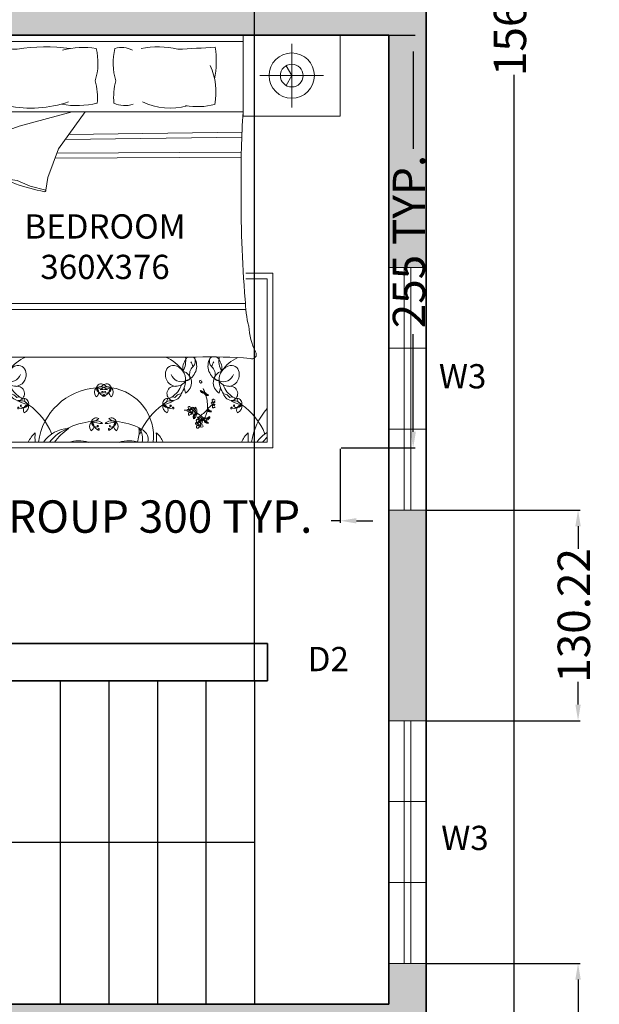
# Model space of a CAD drawing. Units: centimetres. Extents: x 2137 to 3697, y 183 to 2094.
# Tile 6 of 8: x 3339 to 3697, y 600 to 1208. Entities that reach past the tile are written whole.
import ezdxf

# ---------------------------------------------------------------- set-up
doc = ezdxf.new("R2010")
doc.units = ezdxf.units.CM
for name, color, linetype, lineweight in [('A-ANNO-DIMS', 2, 'Continuous', 18), ('A-ANNO-TEXT', 7, 'Continuous', 18), ('A-AREA-IDEN', 7, 'Continuous', 25), ('A-FLOR-STRS', 7, 'Continuous', 25), ('A-FURN', 8, 'Continuous', 18), ('A-GLAZ', 4, 'Continuous', 18), ('A-WALL', 7, 'Continuous', 35), ('A-WALL-PATT', 52, 'Continuous', 13)]:
    doc.layers.add(name, color=color, linetype=linetype, lineweight=lineweight)
doc.styles.get("Standard").update_dxf_attribs({"font": 'arial.ttf'})
doc.dimstyles.new('ISO-25', dxfattribs={"dimtxt": 20, "dimasz": 10, "dimexe": 1.25, "dimexo": 0.625, "dimtad": 0, "dimtxsty": 'Standard', "dimcen": 2.5, "dimadec": 0, "dimazin": 0, "dimtfac": 1, "dimtmove": 0, "dimatfit": 3, "dimfxl": 1, "dimarcsym": 0})

# ---------------------------------------------------------------- blocks, each defined once
blk = doc.blocks.new('*D3')
at = {"layer": 'A-ANNO-DIMS', "color": 0, "lineweight": -2, "transparency": 16777216}
for p, q in [((3590.65, 1986.58), (3645.66, 1986.58)), ((3644.41, 1976.58), (3644.41, 1233.12)), ((3644.41, 430.58), (3644.41, 1174.04)), ((3590.65, 420.58), (3645.66, 420.58))]:
    blk.add_line(p, q, dxfattribs=at)
at = {"layer": 'A-ANNO-DIMS', "color": 0, "transparency": 16777216}
for points in [[(3642.74, 1976.58), (3646.07, 1976.58), (3644.41, 1986.58)], [(3642.74, 430.58), (3646.07, 430.58), (3644.41, 420.58)]]:
    blk.add_solid(points, dxfattribs=at)
at = {"layer": 'Defpoints', "color": 0, "transparency": 16777216}
for p in [(3590.02, 1986.58), (3644.41, 1986.58), (3590.02, 420.58)]:
    blk.add_point(p, dxfattribs=at)
at = {"layer": 'A-ANNO-DIMS', "color": 0, "transparency": 16777216, "insert": (3644.41, 1203.58), "char_height": 20, "attachment_point": 5, "rotation": 90}
blk.add_mtext('1566', dxfattribs=at)
blk = doc.blocks.new('BED')
for p, q in [((2442.52, 2474.71), (2742.52, 2474.71)), ((2502.52, 2474.71), (2502.52, 2392.37)), ((2682.52, 2470.86), (2502.52, 2470.86)), ((2472.52, 2430.11), (2472.52, 2469.31)), ((2712.52, 2430.11), (2712.52, 2469.31)), ((2492.12, 2449.71), (2452.92, 2449.71)), ((2692.92, 2449.71), (2732.12, 2449.71)), ((2502.52, 2427.3), (2682.52, 2427.3)), ((2544.19, 2418.38), (2576.9, 2427.3)), ((2584.93, 2427.3), (2568.49, 2404.42)), ((2522.31, 2410.49), (2544.19, 2418.38)), ((2510.77, 2401.99), (2522.31, 2410.49)), ((2681.6, 2411.76), (2572.66, 2410.22)), ((2681.71, 2414.84), (2574.9, 2413.34)), ((2568.49, 2404.42), (2561.81, 2386.81)), ((2499.83, 2389.24), (2510.77, 2401.99)), ((2681.46, 2399.23), (2566.35, 2398.76)), ((2681.44, 2402.31), (2567.52, 2401.86)), ((2502.26, 2386.81), (2499.83, 2389.24)), ((2514.41, 2388.02), (2502.26, 2386.81)), ((2529.61, 2386.81), (2514.41, 2388.02)), ((2542.97, 2384.99), (2529.61, 2386.81)), ((2561.81, 2386.81), (2560.59, 2378.91)), ((2550.87, 2381.34), (2542.97, 2384.99)), ((2560.59, 2378.91), (2550.87, 2381.34)), ((2482.11, 2327.65), (2499.08, 2327.65)), ((2482.11, 2219.58), (2482.11, 2327.65)), ((2684.19, 2327.65), (2700.83, 2327.65)), ((2700.83, 2327.65), (2700.83, 2219.58)), ((2499.08, 2324.17), (2485.59, 2324.17)), ((2485.59, 2324.17), (2485.59, 2223.06)), ((2697.35, 2324.17), (2684.13, 2324.17)), ((2697.35, 2223.06), (2697.35, 2324.17)), ((2683.88, 2308.94), (2499.06, 2308.94)), ((2684.17, 2305.2), (2499.06, 2305.2)), ((2653.42, 2275.73), (2531.62, 2275.73)), ((2515.15, 2253.47), (2514.49, 2256.86)), ((2536.12, 2253.47), (2536.78, 2256.86)), ((2646.82, 2253.47), (2646.16, 2256.86)), ((2667.79, 2253.47), (2668.45, 2256.86)), ((2485.59, 2223.06), (2697.35, 2223.06)), ((2700.83, 2219.58), (2482.11, 2219.58))]:
    blk.add_line(p, q)
for points in [[(2502.52, 2424.71), (2442.52, 2424.71), (2442.52, 2474.71)], [(2682.52, 2474.71), (2682.52, 2424.71), (2742.52, 2424.71), (2742.52, 2474.71)], [(2472.52, 2449.71), (2476.02, 2455.77)], [(2712.52, 2449.71), (2709.02, 2455.77)], [(2472.52, 2449.71), (2476.02, 2443.65)], [(2712.52, 2449.71), (2709.02, 2443.65)]]:
    blk.add_lwpolyline(points)
for points in [[(2519.75, 2467.23, 0.074897), (2520.11, 2447.64, -0.472817)], [(2591.11, 2446.54, 0.14099), (2591.71, 2466.53, 0.235245)], [(2603.92, 2446.54, -0.14099), (2603.32, 2466.53, -0.235245)], [(2665.29, 2467.23, -0.074897), (2664.92, 2447.64, 0.472817)], [(2499.2, 2361.77, 0.001242), (2499.06, 2304.85, -0.127202), (2493.05, 2276.48)], [(2683.8, 2311.3, 0.056112), (2685.97, 2294.79, 0.095341), (2690.19, 2278.9)]]:
    blk.add_lwpolyline(points, format="xyb")
for centre, radius in [((2472.52, 2449.71), 14), ((2712.52, 2449.71), 14), ((2472.52, 2449.71), 7), ((2712.52, 2449.71), 7), ((2532.49, 2242.6), 0.764), ((2650.46, 2242.6), 0.764), ((2527.49, 2234.55), 0.764), ((2655.45, 2234.55), 0.764)]:
    blk.add_circle(centre, radius)
for centre, radius, start, end in [((2685.11, 5322.24), 2859.79, 266.68521, 267.14978), ((2560.85, 2358.67), 108.8, 82.21958, 99.49698), ((2583.83, 2413.66), 53.46, 81.52493, 103.95996), ((2607.44, 2452.27), 14.84, 63.34374, 106.10256), ((2629.68, 2414.74), 52.74, 76.34271, 101.1841), ((2499.93, 5322.24), 2859.79, 272.85022, 273.31479), ((2557.97, 2439.77), 38.67, 155.1316, 191.75834), ((2627.07, 2439.77), 38.67, 348.24166, 24.8684), ((2555.75, 2436.51), 36.76, 354.01289, 15.82928), ((2639.29, 2436.51), 36.76, 164.17072, 185.98711), ((2530.45, 2470.74), 40.2, 255.10393, 281.03689), ((2551.61, 2499.32), 69.73, 258.03974, 289.26152), ((2579.84, 2484.1), 52.9, 259.86169, 283.62376), ((2609.45, 2447.1), 15.9, 245.01826, 288.54073), ((2637.23, 2467.78), 38.19, 243.87611, 286.17464), ((2654.58, 2470.74), 40.2, 258.96311, 284.89607), ((3220.32, 2390.64), 539.05, 176.09997, 180.92818), ((2224.76, 2381.78), 275.17, 355.82941, 1.55305), ((2504.97, 2495.47), 113.22, 267.45188, 281.3392), ((2532.03, 2360.52), 24.42, 66.26158, 101.3392), ((2581.42, 2492.28), 116.34, 250.11942, 259.33829), ((3384.42, 2371.04), 703.17, 179.11454, 184.87351), ((2559.91, 2378.67), 0.724, 268.86235, 19.75363), ((2495.81, 2276.67), 2.77, 183.97998, 297.34124), ((2687.92, 2277.37), 2.73, 246.52186, 33.82642), ((2528.04, 1963.45), 312.3, 89.34325, 95.68869), ((2507.86, 2265.5), 5.07, 84.48557, 181.05378), ((2494.64, 2254.6), 22.71, 33.66712, 63.29966), ((2506.31, 2261.76), 9.02, 355.29334, 76.921), ((2525.07, 2268.11), 11.57, 145.78505, 184.73037), ((2502.97, 2273.51), 12.43, 328.82178, 9.15542), ((2518.36, 2272.41), 3.61, 120.0293, 142.32497), ((2512.59, 2270.28), 9.56, 289.28218, 29.1751), ((2511.15, 2268.55), 8.62, 7.43599, 29.91487), ((2516.83, 2273.13), 4.49, 311.56531, 23.83541), ((2518.36, 2272.41), 3.61, 44.45169, 63.55801), ((2538.68, 2270.28), 9.56, 150.8249, 250.71782), ((2534.44, 2273.13), 4.49, 156.16459, 228.43469), ((2532.91, 2272.41), 3.61, 113.22901, 135.54831), ((2540.13, 2268.55), 8.62, 150.08513, 172.56401), ((2532.91, 2272.41), 3.61, 37.67503, 66.71436), ((2526.21, 2268.11), 11.57, 355.26963, 34.21495), ((2548.31, 2273.51), 12.43, 169.71335, 211.17822), ((2544.97, 2261.76), 9.02, 103.079, 184.70666), ((2556.64, 2254.6), 22.71, 111.49413, 146.33288), ((2543.41, 2265.5), 5.07, 358.94622, 95.51443), ((2639.53, 2265.5), 5.07, 84.48557, 181.05378), ((2626.3, 2254.6), 22.71, 33.66712, 68.50587), ((2637.98, 2261.76), 9.02, 355.29334, 76.921), ((2656.73, 2268.11), 11.57, 145.78505, 184.73037), ((2634.63, 2273.51), 12.43, 328.82178, 10.28665), ((2650.03, 2272.41), 3.61, 113.28564, 142.32497), ((2644.26, 2270.28), 9.56, 289.28218, 29.1751), ((2642.81, 2268.55), 8.62, 7.43599, 29.91487), ((2650.03, 2272.41), 3.61, 44.45169, 66.71436), ((2648.5, 2273.13), 4.49, 311.56531, 23.83541), ((2662.61, 1983.95), 291.92, 85.24024, 91.80351), ((2670.35, 2270.28), 9.56, 150.8249, 250.71782), ((2666.11, 2273.13), 4.49, 156.16459, 228.43469), ((2664.58, 2272.41), 3.61, 106.63434, 135.54831), ((2671.79, 2268.55), 8.62, 150.08513, 172.56401), ((2664.58, 2272.41), 3.61, 37.67503, 72.58143), ((2657.87, 2268.11), 11.57, 355.26963, 34.21495), ((2679.98, 2273.51), 12.43, 169.24899, 211.17822), ((2676.63, 2261.76), 9.02, 103.079, 184.70666), ((2688.3, 2254.6), 22.71, 113.64533, 146.33288), ((2675.08, 2265.5), 5.07, 358.94622, 95.51443), ((2509.94, 2264.78), 7.17, 174.94485, 262.88575), ((2512.76, 2267.5), 6.96, 201.58187, 291.42215), ((2511.44, 2259.94), 7.46, 299.90854, 73.1337), ((2523.89, 2265.16), 6.15, 131.56531, 195.14713), ((2527.38, 2265.16), 6.15, 344.85287, 48.43469), ((2539.84, 2259.94), 7.46, 106.8663, 240.09146), ((2538.52, 2267.5), 6.96, 248.57785, 338.41813), ((2541.33, 2264.78), 7.17, 277.11425, 5.05515), ((2641.61, 2264.78), 7.17, 174.94485, 262.88575), ((2644.43, 2267.5), 6.96, 201.58187, 291.42215), ((2643.1, 2259.94), 7.46, 299.90854, 73.1337), ((2655.56, 2265.16), 6.15, 131.56531, 195.14713), ((2659.05, 2265.16), 6.15, 344.85287, 48.43469), ((2671.51, 2259.94), 7.46, 106.8663, 240.09146), ((2670.18, 2267.5), 6.96, 248.57785, 338.41813), ((2673, 2264.78), 7.17, 277.11425, 5.05515), ((2499.37, 2263.14), 14.16, 301.26137, 341.7045), ((2508.7, 2266.37), 8.71, 272.3591, 324.04014), ((2499.23, 2262), 16.1, 326.28828, 356.5076), ((2525.07, 2268.11), 11.57, 212.70113, 216.34448), ((2516.16, 2263.07), 1.86, 257.30406, 15.14713), ((2526.5, 2260.25), 0.578, 102.70507, 280.43845), ((2526.43, 2260.6), 0.94, 280.43845, 100.41356), ((2535.12, 2263.07), 1.86, 164.85287, 282.69594), ((2526.21, 2268.11), 11.57, 323.65552, 327.29887), ((2542.58, 2266.37), 8.71, 215.95986, 267.6409), ((2552.04, 2262), 16.1, 183.4924, 213.71172), ((2551.91, 2263.14), 14.16, 198.2955, 238.73863), ((2594.92, 2255.93), 3.25, 63.02737, 163.80375), ((2591.63, 2263.52), 6.69, 271.45846, 315.37266), ((2598.02, 2255.93), 3.25, 16.19625, 116.97263), ((2601.31, 2263.52), 6.69, 224.62734, 268.54154), ((2631.03, 2263.14), 14.16, 301.26137, 341.7045), ((2640.36, 2266.37), 8.71, 272.3591, 324.04014), ((2630.9, 2262), 16.1, 326.28828, 356.5076), ((2656.73, 2268.11), 11.57, 212.70113, 216.34448), ((2647.82, 2263.07), 1.86, 257.30406, 15.14713), ((2656.51, 2260.6), 0.94, 79.58644, 259.56155), ((2656.44, 2260.25), 0.578, 259.56155, 77.29493), ((2666.78, 2263.07), 1.86, 164.85287, 282.69594), ((2657.87, 2268.11), 11.57, 323.65552, 327.29887), ((2674.25, 2266.37), 8.71, 215.95986, 267.6409), ((2683.71, 2262), 16.1, 183.4924, 213.71172), ((2683.58, 2263.14), 14.16, 198.2955, 238.73863), ((2508.29, 2253.23), 4.5, 80.26398, 250.86884), ((2507.21, 2254.58), 5.62, 265.96902, 344.3045), ((2513.27, 2247.11), 5.99, 96.1662, 141.58255), ((2523.19, 2251.31), 1.58, 101.32561, 154.46214), ((2520.92, 2256.65), 4.74, 280.25878, 300.65599), ((2522.01, 2260.45), 8.46, 268.32639, 277.13024), ((2547.29, 2245.15), 24.85, 163.58418, 183.82768), ((2519.89, 2256.64), 4.82, 308.21012, 316.30712), ((2522.85, 2253.47), 1.44, 278.34322, 4.28685), ((2522.06, 2254.74), 2.51, 300.65599, 332.63414), ((2523.94, 2253.08), 0.611, 55.76575, 157.44165), ((2547.29, 2245.15), 24.85, 153.0032, 159.89408), ((2524.9, 2253.65), 0.611, 84.37838, 186.05427), ((2524.32, 2256.1), 2.51, 269.18588, 301.16403), ((2525.06, 2254.8), 1.44, 237.53317, 323.47681), ((2523.67, 2258.9), 4.82, 285.51291, 293.60991), ((2526.81, 2253.48), 1.58, 87.35788, 140.49441), ((2523.17, 2258), 4.74, 301.16403, 321.56124), ((2519.31, 2258.83), 8.46, 324.68979, 333.49364), ((2538.01, 2247.11), 5.99, 38.41745, 83.8338), ((2544.06, 2254.58), 5.62, 195.6955, 274.03098), ((2542.98, 2253.23), 4.5, 289.13116, 99.73602), ((2594.85, 2217.78), 39.18, 94.46233, 172.25504), ((2595.02, 2253.92), 4.34, 137.78732, 219.11446), ((2590.09, 2254.05), 3.27, 298.5391, 58.36268), ((2594.35, 2251.19), 6.19, 45.54113, 114.31008), ((2600, 2282.98), 27.41, 252.59304, 267.25817), ((2595, 2256.71), 3.2, 177.75849, 283.85198), ((2601.17, 2260.05), 9.91, 198.91595, 238.01098), ((2598.59, 2251.19), 6.19, 65.68992, 134.45887), ((2592.94, 2282.98), 27.41, 272.74183, 287.40696), ((2595.67, 2254.01), 0.424, 283.85198, 219.92454), ((2596.18, 2252.06), 0.487, 238.01098, 71.55918), ((2596.26, 2252.29), 0.236, 71.55918, 188.01668), ((2596.76, 2252.06), 0.487, 108.44082, 301.98902), ((2596.68, 2252.29), 0.236, 351.98332, 108.44082), ((2597.23, 2254.17), 0.255, 320.19092, 256.02088), ((2591.77, 2260.05), 9.91, 301.98902, 341.08405), ((2597.94, 2256.71), 3.2, 256.14802, 2.24151), ((2602.86, 2254.05), 3.27, 121.63732, 241.4609), ((2597.92, 2253.92), 4.34, 320.88554, 42.21268), ((2596.83, 2226.82), 30.32, 352.86355, 81.81966), ((2639.96, 2253.23), 4.5, 80.26398, 250.86884), ((2638.88, 2254.58), 5.62, 265.96902, 344.3045), ((2644.93, 2247.11), 5.99, 96.1662, 141.58255), ((2656.13, 2253.48), 1.58, 39.50559, 92.64212), ((2659.77, 2258), 4.74, 218.43876, 238.83597), ((2663.63, 2258.83), 8.46, 206.50636, 215.31021), ((2657.88, 2254.8), 1.44, 216.52319, 302.46683), ((2658.62, 2256.1), 2.51, 238.83597, 270.81412), ((2659.27, 2258.9), 4.82, 246.39009, 254.48709), ((2635.65, 2245.15), 24.85, 20.10592, 26.9968), ((2658.05, 2253.65), 0.611, 353.94573, 95.62162), ((2659, 2253.08), 0.611, 22.55835, 124.23425), ((2660.09, 2253.47), 1.44, 175.71315, 261.65678), ((2660.89, 2254.74), 2.51, 207.36586, 239.34401), ((2635.65, 2245.15), 24.85, 356.17232, 16.41582), ((2663.05, 2256.64), 4.82, 223.69288, 231.78988), ((2662.02, 2256.65), 4.74, 239.34401, 259.74122), ((2660.93, 2260.45), 8.46, 262.86976, 271.67361), ((2659.76, 2251.31), 1.58, 25.53786, 78.67439), ((2675.73, 2254.58), 5.62, 195.6955, 274.03098), ((2669.67, 2247.11), 5.99, 38.41745, 83.8338), ((2674.65, 2253.23), 4.5, 289.13116, 99.73602), ((2523.45, 2213.9), 39.18, 124.38655, 158.59079), ((2505.57, 2245.31), 4.34, 167.71153, 249.03868), ((2504.48, 2247), 3.25, 92.95159, 193.72796), ((2497.84, 2251.95), 6.69, 301.38267, 345.29688), ((2506.35, 2242.61), 6.19, 75.46535, 144.23429), ((2495.38, 2272.99), 27.41, 282.51726, 297.18239), ((2501.23, 2242.96), 3.27, 328.46331, 88.28689), ((2507.84, 2253.69), 9.91, 228.84017, 267.9352), ((2504.16, 2247.72), 3.2, 207.6827, 313.77619), ((2507.37, 2248.35), 2.76, 63.97555, 143.26805), ((2506.09, 2245.71), 0.424, 313.77619, 249.71835), ((2518.73, 2248.32), 1.27, 101.56373, 142.6358), ((2517.68, 2247.14), 0.764, 273.27684, 86.72316), ((2518.57, 2247.86), 0.73, 91.10805, 181.86747), ((2520.08, 2247.41), 2.32, 203.42757, 227.61037), ((2519.34, 2246.4), 1.58, 80.3487, 133.65382), ((2519.06, 2247.7), 1.25, 229.78892, 317.67915), ((2517.71, 2249.32), 1.84, 288.72627, 352.50315), ((2517.65, 2245.06), 1.78, 355.05304, 68.36176), ((2519.04, 2244.75), 2.5, 83.08516, 105.71709), ((2518.96, 2249.23), 0.59, 345.23556, 144.9248), ((2501.72, 2224.01), 28.48, 43.15413, 52.0459), ((2519.5, 2247.3), 0.658, 317.67915, 80.3487), ((2543.91, 2248.35), 2.76, 36.73195, 116.02445), ((2544.93, 2242.61), 6.19, 35.76571, 104.53465), ((2555.89, 2272.99), 27.41, 242.81761, 257.48274), ((2543.43, 2253.69), 9.91, 272.0648, 311.15983), ((2547.11, 2247.72), 3.2, 226.22381, 332.3173), ((2545.24, 2245.88), 0.255, 290.26671, 226.22708), ((2550.05, 2242.96), 3.27, 91.71311, 211.53669), ((2546.8, 2247), 3.25, 346.27204, 87.04841), ((2553.44, 2251.95), 6.69, 194.70312, 238.61733), ((2545.71, 2245.31), 4.34, 290.96132, 12.28847), ((2527.83, 2213.9), 39.18, 21.40921, 55.61345), ((2655.12, 2213.9), 39.18, 124.38655, 158.59079), ((2637.23, 2245.31), 4.34, 167.71153, 249.03868), ((2636.14, 2247), 3.25, 92.95159, 193.72796), ((2629.51, 2251.95), 6.69, 301.38267, 345.29688), ((2638.02, 2242.61), 6.19, 75.46535, 144.23429), ((2627.05, 2272.99), 27.41, 282.51726, 297.18239), ((2635.83, 2247.72), 3.2, 207.6827, 313.77619), ((2639.51, 2253.69), 9.91, 228.84017, 267.9352), ((2632.89, 2242.96), 3.27, 328.46331, 88.28689), ((2639.03, 2248.35), 2.76, 63.97555, 143.26805), ((2637.75, 2245.71), 0.424, 313.77619, 249.71835), ((2681.22, 2224.01), 28.48, 127.9541, 136.84587), ((2663.45, 2247.3), 0.658, 99.6513, 222.32085), ((2663.88, 2247.7), 1.25, 222.32085, 310.21108), ((2663.6, 2246.4), 1.58, 46.34618, 99.6513), ((2663.98, 2249.23), 0.59, 35.0752, 194.76444), ((2665.23, 2249.32), 1.84, 187.49685, 251.27373), ((2665.29, 2245.06), 1.78, 111.63824, 184.94696), ((2663.9, 2244.75), 2.5, 74.28291, 96.91484), ((2664.38, 2247.86), 0.73, 358.13253, 88.89195), ((2662.86, 2247.41), 2.32, 312.38963, 336.57243), ((2664.21, 2248.32), 1.27, 37.3642, 78.43627), ((2665.27, 2247.14), 0.764, 93.27684, 266.72316), ((2675.58, 2248.35), 2.76, 36.73195, 116.02445), ((2676.59, 2242.61), 6.19, 35.76571, 104.53465), ((2687.56, 2272.99), 27.41, 242.81761, 257.48274), ((2675.1, 2253.69), 9.91, 272.0648, 311.15983), ((2678.78, 2247.72), 3.2, 226.22381, 332.3173), ((2676.9, 2245.88), 0.255, 290.26671, 226.22708), ((2681.72, 2242.96), 3.27, 91.71311, 211.53669), ((2685.1, 2251.95), 6.69, 194.70312, 238.61733), ((2678.46, 2247), 3.25, 346.27204, 87.04841), ((2677.37, 2245.31), 4.34, 290.96132, 12.28847), ((2659.49, 2213.9), 39.18, 21.40921, 55.61345), ((2456.43, 2217.78), 39.18, 7.74496, 41.8856), ((2507.46, 2244.52), 0.236, 101.4834, 217.94089), ((2507.5, 2244.28), 0.487, 267.9352, 101.4834), ((2518.72, 2245.73), 1.26, 217.76209, 259.04026), ((2518.83, 2244.95), 0.586, 232.47371, 355.05304), ((2521.4, 2241.21), 1.58, 101.32561, 154.46214), ((2519.13, 2246.56), 4.74, 280.25878, 300.65599), ((2520.22, 2250.35), 8.46, 268.32639, 277.13024), ((2518.11, 2246.55), 4.82, 308.21012, 316.30712), ((2521.07, 2243.38), 1.44, 278.34322, 4.28685), ((2520.27, 2244.64), 2.51, 300.65599, 332.63414), ((2522.16, 2242.98), 0.611, 55.76575, 157.44165), ((2534.91, 2244.52), 12.46, 184.75602, 209.20408), ((2552.85, 2271.04), 40.99, 222.24124, 232.17444), ((2536.2, 2227.98), 14.94, 120.54402, 139.81798), ((2528.5, 2242.96), 2.12, 272.84988, 356.12261), ((2526.64, 2243.74), 3.48, 304.53686, 16.36991), ((2527, 2242.14), 2.05, 321.76073, 7.92519), ((2527.43, 2239.19), 2.05, 8.72271, 54.88717), ((2527.54, 2237.55), 3.48, 0.278, 72.11105), ((2531.47, 2242.76), 2.46, 127.31045, 187.92519), ((2529.1, 2238.83), 2.12, 20.5253, 88.5375), ((2528.09, 2243.04), 2.53, 355.01064, 41.65801), ((2530.88, 2241.17), 0.757, 148.0499, 225.62681), ((2536.2, 2227.98), 14.94, 113.05007, 113.84774), ((2532.28, 2240.29), 2.41, 104.75581, 148.0499), ((2530.93, 2242.02), 1.51, 247.40857, 351.43859), ((2531.64, 2243.66), 1.04, 126.10456, 271.42811), ((2528.73, 2238.64), 2.53, 334.9899, 21.63727), ((2531.53, 2243.95), 0.749, 353.75256, 131.70535), ((2531.35, 2241.96), 0.506, 262.90601, 7.13198), ((2530.82, 2243.06), 1.05, 0.06451, 61.15075), ((2531.07, 2243.95), 1.2, 311.84125, 355.78771), ((2533.54, 2243.78), 1.27, 101.56373, 176.36503), ((2533.53, 2241.19), 1.26, 151.21959, 259.04026), ((2533.38, 2243.32), 0.73, 91.10805, 181.86747), ((2534.89, 2242.87), 2.32, 203.42757, 227.61037), ((2534.15, 2241.86), 1.58, 80.3487, 133.65382), ((2533.87, 2243.16), 1.25, 229.78892, 317.67915), ((2532.52, 2244.78), 1.84, 288.72627, 352.50315), ((2532.46, 2240.51), 1.78, 355.05304, 68.36176), ((2533.85, 2240.21), 2.5, 83.08516, 105.71709), ((2533.77, 2244.69), 0.59, 345.23556, 144.9248), ((2533.64, 2240.41), 0.586, 232.47371, 355.05304), ((2534.31, 2242.76), 0.658, 317.67915, 80.3487), ((2536.2, 2227.98), 14.94, 87.10709, 94.75853), ((2543.77, 2244.28), 0.487, 78.5166, 272.0648), ((2543.82, 2244.52), 0.236, 322.05911, 78.5166), ((2639.12, 2244.52), 0.236, 101.4834, 217.94089), ((2639.17, 2244.28), 0.487, 267.9352, 101.4834), ((2646.75, 2227.98), 14.94, 85.24147, 92.89291), ((2648.64, 2242.76), 0.658, 99.6513, 222.32085), ((2649.07, 2243.16), 1.25, 222.32085, 310.21108), ((2648.79, 2241.86), 1.58, 46.34618, 99.6513), ((2649.17, 2244.69), 0.59, 35.0752, 194.76444), ((2650.42, 2244.78), 1.84, 187.49685, 251.27373), ((2650.48, 2240.51), 1.78, 111.63824, 184.94696), ((2649.3, 2240.41), 0.586, 184.94696, 307.52629), ((2649.09, 2240.21), 2.5, 74.28291, 96.91484), ((2649.56, 2243.32), 0.73, 358.13253, 88.89195), ((2648.05, 2242.87), 2.32, 312.38963, 336.57243), ((2649.4, 2243.78), 1.27, 3.63497, 78.43627), ((2649.41, 2241.19), 1.26, 280.95974, 28.78041), ((2652.01, 2242.02), 1.51, 188.56141, 292.59143), ((2651.41, 2243.95), 0.749, 48.29465, 186.24744), ((2651.87, 2243.95), 1.2, 184.21229, 228.15875), ((2652.12, 2243.06), 1.05, 118.84925, 179.93549), ((2651.59, 2241.96), 0.506, 172.86802, 277.09399), ((2651.3, 2243.66), 1.04, 268.57189, 53.89544), ((2650.66, 2240.29), 2.41, 31.9501, 75.24419), ((2654.21, 2238.64), 2.53, 158.36273, 205.0101), ((2653.84, 2238.83), 2.12, 91.4625, 159.4747), ((2655.4, 2237.55), 3.48, 107.88895, 179.722), ((2654.85, 2243.04), 2.53, 138.34199, 184.98936), ((2654.44, 2242.96), 2.12, 183.87739, 267.15012), ((2652.06, 2241.17), 0.757, 314.37319, 31.9501), ((2646.75, 2227.98), 14.94, 66.15226, 66.94993), ((2656.3, 2243.74), 3.48, 163.63009, 235.46314), ((2651.47, 2242.76), 2.46, 352.07481, 52.68955), ((2655.51, 2239.19), 2.05, 125.11283, 171.27729), ((2655.94, 2242.14), 2.05, 172.07481, 218.23927), ((2646.75, 2227.98), 14.94, 40.18202, 59.45598), ((2630.09, 2271.04), 40.99, 307.82556, 317.75876), ((2648.03, 2244.52), 12.46, 330.79592, 355.24398), ((2660.78, 2242.98), 0.611, 22.55835, 124.23425), ((2661.88, 2243.38), 1.44, 175.71315, 261.65678), ((2662.67, 2244.64), 2.51, 207.36586, 239.34401), ((2664.83, 2246.55), 4.82, 223.69288, 231.78988), ((2663.81, 2246.56), 4.74, 239.34401, 259.74122), ((2662.72, 2250.35), 8.46, 262.86976, 271.67361), ((2661.54, 2241.21), 1.58, 25.53786, 78.67439), ((2664.11, 2244.95), 0.586, 184.94696, 307.52629), ((2664.23, 2245.73), 1.26, 280.95974, 322.23791), ((2675.44, 2244.28), 0.487, 78.5166, 272.0648), ((2675.49, 2244.52), 0.236, 322.05911, 78.5166), ((2726.52, 2217.78), 39.18, 138.1144, 172.25504), ((2521.93, 2238.45), 0.853, 146.86359, 236.90213), ((2533.96, 2257.24), 22.32, 235.1882, 238.88441), ((2523.39, 2239.69), 2.31, 199.47987, 267.68284), ((2523.14, 2238.82), 1.99, 212.81548, 277.39917), ((2521.98, 2237.49), 2.31, 266.97007, 338.29129), ((2509.81, 2253.97), 22.32, 302.6784, 306.37461), ((2522.56, 2235.66), 0.853, 214.3538, 304.39233), ((2522.88, 2238.89), 0.883, 238.88441, 314.26458), ((2522.69, 2236.91), 1.99, 280.30568, 17.1958), ((2522.52, 2236.71), 0.883, 306.37461, 21.75478), ((2523.96, 2237.28), 0.666, 19.36054, 201.75478), ((2523.96, 2237.78), 0.666, 311.87034, 134.26458), ((2536.49, 2231.71), 13.31, 153.78194, 158.29129), ((2525.9, 2240.8), 3.48, 247.23048, 319.06353), ((2524.75, 2239.63), 2.05, 264.45436, 310.61881), ((2534.91, 2244.52), 12.46, 214.00334, 222.49171), ((2526.25, 2238.81), 2.12, 218.32082, 298.81623), ((2525.88, 2233.11), 0.757, 148.0499, 225.62681), ((2527.28, 2232.24), 2.41, 104.75581, 148.0499), ((2525.93, 2233.96), 1.51, 247.40857, 351.43859), ((2526.65, 2235.61), 1.04, 126.10456, 271.42811), ((2526.53, 2235.89), 0.749, 353.75256, 131.70535), ((2527.69, 2236.2), 2.46, 70.00407, 130.61881), ((2526.36, 2233.9), 0.506, 262.90601, 7.13198), ((2525.83, 2235), 1.05, 0.06451, 61.15075), ((2526.08, 2235.9), 1.2, 311.84125, 355.78771), ((2526.09, 2239.2), 2.53, 297.70426, 344.35163), ((2528.55, 2235.73), 1.27, 101.56373, 176.36503), ((2528.53, 2233.13), 1.26, 151.21959, 259.04026), ((2528.38, 2235.27), 0.73, 91.10805, 181.86747), ((2529.89, 2234.81), 2.32, 203.42757, 227.61037), ((2529.15, 2233.8), 1.58, 80.3487, 133.65382), ((2528.87, 2235.11), 1.25, 229.78892, 317.67915), ((2527.52, 2236.73), 1.84, 288.72627, 352.50315), ((2527.46, 2232.46), 1.78, 355.05304, 68.36176), ((2528.85, 2232.16), 2.5, 83.08516, 105.71709), ((2528.77, 2236.64), 0.59, 345.23556, 144.9248), ((2529.31, 2234.71), 0.658, 317.67915, 80.3487), ((2531.89, 2239.88), 2.46, 188.72271, 249.33746), ((2591.85, 2196.79), 39.18, 94.46233, 117.4146), ((2592.02, 2232.93), 4.34, 137.78732, 219.11446), ((2587.09, 2233.07), 3.27, 298.5391, 58.36268), ((2591.92, 2234.94), 3.25, 63.02737, 163.80375), ((2588.63, 2242.54), 6.69, 271.45846, 315.37266), ((2591.35, 2230.21), 6.19, 45.54113, 114.31008), ((2598.17, 2239.06), 9.91, 198.91595, 238.01098), ((2597, 2262), 27.41, 252.59304, 267.25817), ((2592, 2235.73), 3.2, 177.75849, 283.85198), ((2601.59, 2230.21), 6.19, 65.68992, 134.45887), ((2595.94, 2262), 27.41, 272.74183, 287.40696), ((2601.02, 2234.94), 3.25, 16.19625, 116.97263), ((2604.31, 2242.54), 6.69, 224.62734, 268.54154), ((2594.77, 2239.06), 9.91, 301.98902, 341.08405), ((2600.94, 2235.73), 3.2, 256.14802, 2.24151), ((2605.86, 2233.07), 3.27, 121.63732, 241.4609), ((2600.92, 2232.93), 4.34, 320.88554, 42.21268), ((2601.09, 2196.79), 39.18, 62.5854, 85.53767), ((2651.05, 2239.88), 2.46, 290.66254, 351.27729), ((2653.63, 2234.71), 0.658, 99.6513, 222.32085), ((2654.07, 2235.11), 1.25, 222.32085, 310.21108), ((2653.79, 2233.8), 1.58, 46.34618, 99.6513), ((2654.17, 2236.64), 0.59, 35.0752, 194.76444), ((2655.42, 2236.73), 1.84, 187.49685, 251.27373), ((2655.48, 2232.46), 1.78, 111.63824, 184.94696), ((2654.09, 2232.16), 2.5, 74.28291, 96.91484), ((2655.26, 2236.2), 2.46, 49.38119, 109.99593), ((2657.04, 2240.8), 3.48, 220.93647, 292.76952), ((2656.85, 2239.2), 2.53, 195.64837, 242.29574), ((2654.56, 2235.27), 0.73, 358.13253, 88.89195), ((2653.05, 2234.81), 2.32, 312.38963, 336.57243), ((2654.4, 2235.73), 1.27, 3.63497, 78.43627), ((2654.41, 2233.13), 1.26, 280.95974, 28.78041), ((2657.01, 2233.96), 1.51, 188.56141, 292.59143), ((2656.41, 2235.89), 0.749, 48.29465, 186.24744), ((2656.69, 2238.81), 2.12, 241.18377, 321.67918), ((2656.87, 2235.9), 1.2, 184.21229, 228.15875), ((2657.12, 2235), 1.05, 118.84925, 179.93549), ((2656.58, 2233.9), 0.506, 172.86802, 277.09399), ((2656.3, 2235.61), 1.04, 268.57189, 53.89544), ((2655.66, 2232.24), 2.41, 31.9501, 75.24419), ((2658.19, 2239.63), 2.05, 229.38119, 275.54564), ((2648.03, 2244.52), 12.46, 317.50829, 325.99666), ((2657.06, 2233.11), 0.757, 314.37319, 31.9501), ((2660.25, 2236.91), 1.99, 162.8042, 259.69432), ((2658.98, 2237.78), 0.666, 45.73542, 228.12966), ((2658.98, 2237.28), 0.666, 338.24522, 160.63946), ((2646.45, 2231.71), 13.31, 21.70871, 26.21806), ((2660.96, 2237.49), 2.31, 201.70871, 273.02993), ((2660.06, 2238.89), 0.883, 225.73542, 301.11559), ((2660.42, 2236.71), 0.883, 158.24522, 233.62539), ((2659.81, 2238.82), 1.99, 262.60083, 327.18452), ((2659.55, 2239.69), 2.31, 272.31716, 340.52013), ((2673.14, 2253.97), 22.32, 233.62539, 237.3216), ((2660.38, 2235.66), 0.853, 235.60767, 325.6462), ((2648.98, 2257.24), 22.32, 301.11559, 304.8118), ((2661.01, 2238.45), 0.853, 303.09787, 33.13641), ((2476.08, 2212.53), 19.09, 33.46172, 60.11157), ((2486.77, 2216.95), 15.93, 22.55474, 48.95456), ((2443.14, 2225.51), 54.2, 357.40811, 3.65191), ((2528.65, 2232.36), 0.586, 232.47371, 355.05304), ((2564.51, 2216.95), 15.93, 131.04544, 157.44526), ((2608.14, 2225.51), 54.2, 176.34809, 182.59189), ((2575.2, 2212.53), 19.09, 91.27197, 146.53828), ((2582.06, 2208.97), 23.79, 107.85038, 143.69643), ((2594.57, 2202.28), 35.39, 124.01234, 144.05304), ((2592.67, 2233.03), 0.424, 283.85198, 219.92454), ((2593.18, 2231.07), 0.487, 238.01098, 71.55918), ((2593.26, 2231.31), 0.236, 71.55918, 188.01668), ((2599.76, 2231.07), 0.487, 108.44082, 301.98902), ((2599.68, 2231.31), 0.236, 351.98332, 108.44082), ((2600.23, 2233.19), 0.255, 320.19092, 256.02088), ((2600.75, 2229.59), 17.54, 338.11703, 6.61954), ((2616.84, 2224.71), 7.03, 346.38982, 79.07385), ((2611.55, 2225.68), 8.89, 342.86088, 41.90487), ((2574.8, 2225.51), 54.2, 357.40811, 3.65191), ((2618.44, 2216.95), 15.93, 22.55474, 48.95456), ((2654.29, 2232.36), 0.586, 184.94696, 307.52629), ((2696.17, 2216.95), 15.93, 131.04544, 157.44526), ((2739.8, 2225.51), 54.2, 176.34809, 182.59189), ((2706.86, 2212.53), 19.09, 119.88843, 146.53828), ((2469.21, 2208.97), 23.79, 36.30357, 46.48142), ((2580.89, 2202.46), 21.54, 73.54311, 107.0202), ((2589.43, 2191.36), 31.85, 94.37872, 95.63574), ((2606.21, 2169.53), 56.92, 109.72171, 109.90284), ((2612.05, 2202.46), 21.54, 72.9798, 106.45689), ((2603.51, 2191.36), 31.85, 84.36426, 85.62128), ((2586.74, 2169.53), 56.92, 70.09716, 70.27829), ((2713.73, 2208.97), 23.79, 133.51858, 143.69643)]:
    blk.add_arc(centre, radius, start, end)
blk = doc.blocks.new('WIN-W3-150CM')
for p, q in [((0, 23), (0, 0)), ((50, 23), (50, 0)), ((100, 23), (100, 0)), ((150, 23), (150, 0)), ((0, 13.5), (150, 13.5)), ((0, 9.5), (150, 9.5))]:
    blk.add_line(p, q)
blk = doc.blocks.new('*D26')
at = {"layer": 'A-ANNO-DIMS', "color": 0, "lineweight": -2, "transparency": 16777216}
for p, q in [((3237.02, 942.82), (3237.02, 897.2)), ((3537.02, 942.82), (3537.02, 897.2)), ((3227.02, 898.45), (3217.02, 898.45)), ((3237.02, 898.45), (3242.68, 898.45)), ((3537.02, 898.45), (3531.37, 898.45)), ((3547.02, 898.45), (3557.02, 898.45))]:
    blk.add_line(p, q, dxfattribs=at)
at = {"layer": 'A-ANNO-DIMS', "color": 0, "transparency": 16777216}
for points in [[(3227.02, 900.12), (3227.02, 896.78), (3237.02, 898.45)], [(3547.02, 900.12), (3547.02, 896.78), (3537.02, 898.45)]]:
    blk.add_solid(points, dxfattribs=at)
at = {"layer": 'Defpoints', "color": 0, "transparency": 16777216}
for p in [(3237.02, 943.45), (3537.02, 943.45), (3537.02, 898.45)]:
    blk.add_point(p, dxfattribs=at)
at = {"layer": 'A-ANNO-DIMS', "color": 0, "transparency": 16777216, "insert": (3387.02, 898.45), "char_height": 20, "attachment_point": 5}
blk.add_mtext('BED GROUP 300 TYP.', dxfattribs=at)
blk = doc.blocks.new('*D27')
at = {"layer": 'A-ANNO-DIMS', "color": 0, "lineweight": -2, "transparency": 16777216}
for p, q in [((3537.65, 1198.58), (3583.27, 1198.58)), ((3582.02, 1188.58), (3582.02, 1128.26)), ((3582.02, 953.45), (3582.02, 1013.77)), ((3537.65, 943.45), (3583.27, 943.45))]:
    blk.add_line(p, q, dxfattribs=at)
at = {"layer": 'A-ANNO-DIMS', "color": 0, "transparency": 16777216}
for points in [[(3580.36, 1188.58), (3583.69, 1188.58), (3582.02, 1198.58)], [(3580.36, 953.45), (3583.69, 953.45), (3582.02, 943.45)]]:
    blk.add_solid(points, dxfattribs=at)
at = {"layer": 'Defpoints', "color": 0, "transparency": 16777216}
for p in [(3537.02, 1198.58), (3582.02, 1198.58), (3537.02, 943.45)]:
    blk.add_point(p, dxfattribs=at)
at = {"layer": 'A-ANNO-DIMS', "color": 0, "transparency": 16777216, "insert": (3582.02, 1071.01), "char_height": 20, "attachment_point": 5, "rotation": 90}
blk.add_mtext('255 TYP.', dxfattribs=at)
blk = doc.blocks.new('*D43')
at = {"layer": 'A-ANNO-DIMS', "color": 0, "lineweight": -2, "transparency": 16777216}
for p, q in [((3184.02, 800.2), (3184.02, 2081.68)), ((3484.02, 800.2), (3484.02, 2081.68)), ((3194.02, 2080.43), (3311.34, 2080.43)), ((3474.02, 2080.43), (3356.7, 2080.43))]:
    blk.add_line(p, q, dxfattribs=at)
at = {"layer": 'A-ANNO-DIMS', "color": 0, "transparency": 16777216}
for points in [[(3194.02, 2082.1), (3194.02, 2078.76), (3184.02, 2080.43)], [(3474.02, 2082.1), (3474.02, 2078.76), (3484.02, 2080.43)]]:
    blk.add_solid(points, dxfattribs=at)
at = {"layer": 'Defpoints', "color": 0, "transparency": 16777216}
for p in [(3484.02, 2080.43), (3184.02, 799.58), (3484.02, 799.58)]:
    blk.add_point(p, dxfattribs=at)
at = {"layer": 'A-ANNO-DIMS', "color": 0, "transparency": 16777216, "insert": (3334.02, 2080.43), "char_height": 20, "attachment_point": 5}
blk.add_mtext('300', dxfattribs=at)
blk = doc.blocks.new('*D45')
at = {"layer": 'A-ANNO-DIMS', "color": 0, "lineweight": -2, "transparency": 16777216}
for p, q in [((3590.65, 624.85), (3685.12, 624.85)), ((3683.87, 614.85), (3683.87, 565.03)), ((3683.87, 430.58), (3683.87, 480.41)), ((3590.65, 420.58), (3685.12, 420.58))]:
    blk.add_line(p, q, dxfattribs=at)
at = {"layer": 'A-ANNO-DIMS', "color": 0, "transparency": 16777216}
for points in [[(3682.21, 614.85), (3685.54, 614.85), (3683.87, 624.85)], [(3682.21, 430.58), (3685.54, 430.58), (3683.87, 420.58)]]:
    blk.add_solid(points, dxfattribs=at)
at = {"layer": 'Defpoints', "color": 0, "transparency": 16777216}
for p in [(3590.02, 624.85), (3590.02, 420.58), (3683.87, 420.58)]:
    blk.add_point(p, dxfattribs=at)
at = {"layer": 'A-ANNO-DIMS', "color": 0, "transparency": 16777216, "insert": (3683.87, 522.72), "char_height": 20, "attachment_point": 5, "rotation": 90}
blk.add_mtext('204.27', dxfattribs=at)
blk = doc.blocks.new('*D46')
at = {"layer": 'A-ANNO-DIMS', "color": 0, "lineweight": -2, "transparency": 16777216}
for p, q in [((3590.65, 905.08), (3685.12, 905.08)), ((3683.87, 895.08), (3683.87, 881.06)), ((3683.87, 784.85), (3683.87, 798.87)), ((3590.65, 774.85), (3685.12, 774.85))]:
    blk.add_line(p, q, dxfattribs=at)
at = {"layer": 'A-ANNO-DIMS', "color": 0, "transparency": 16777216}
for points in [[(3682.21, 895.08), (3685.54, 895.08), (3683.87, 905.08)], [(3682.21, 784.85), (3685.54, 784.85), (3683.87, 774.85)]]:
    blk.add_solid(points, dxfattribs=at)
at = {"layer": 'Defpoints', "color": 0, "transparency": 16777216}
for p in [(3590.02, 905.08), (3590.02, 774.85), (3683.87, 774.85)]:
    blk.add_point(p, dxfattribs=at)
at = {"layer": 'A-ANNO-DIMS', "color": 0, "transparency": 16777216, "insert": (3683.87, 839.96), "char_height": 20, "attachment_point": 5, "rotation": 90}
blk.add_mtext('130.22', dxfattribs=at)

msp = doc.modelspace()

# ---------------------------------------------------------------- hatches: boundary and pattern name
at = {"layer": 'A-WALL-PATT'}
h = msp.add_hatch(color=256, dxfattribs=at)
h.dxf.hatch_style = 1
h.paths.add_polyline_path([(2413.023, 1526.579), (2270.023, 1526.579), (2270.023, 1413.579), (2293.023, 1413.579), (2293.023, 1503.579), (2413.023, 1503.579)])
h.paths.add_polyline_path([(2744.523, 1526.579), (2563.023, 1526.579), (2563.023, 1503.579), (2638.023, 1503.579), (2683.023, 1503.579), (2683.023, 1296.579), (2706.023, 1296.579), (2706.023, 1503.579), (2744.523, 1503.579)])
h.paths.add_polyline_path([(2881.023, 1541.602), (2858.023, 1541.602), (2858.023, 1526.579), (2819.523, 1526.579), (2819.523, 1503.579), (2858.023, 1503.579), (2858.023, 1311.579), (2781.023, 1311.579), (2781.023, 1296.579), (2858.023, 1296.579), (2858.023, 1273.579), (2881.023, 1273.579)])
h.paths.add_polyline_path([(3207.023, 1745.579), (2881.023, 1745.579), (2881.023, 1963.579), (2913.523, 1963.579), (2913.523, 1986.579), (2858.023, 1986.579), (2858.023, 1691.602), (2881.023, 1691.602), (2881.023, 1722.579), (3184.023, 1722.579), (3184.023, 1321.579), (3207.023, 1321.579)])
h.paths.add_polyline_path([(3072.523, 1986.579), (2988.523, 1986.579), (2988.523, 1963.579), (3021.023, 1963.579), (3021.023, 1820.579), (3036.023, 1820.579), (3036.023, 1963.579), (3072.523, 1963.579)], flags=17)
h.paths.add_polyline_path([(3207.023, 1986.579), (3147.523, 1986.579), (3147.523, 1963.579), (3184.023, 1963.579), (3184.023, 1845.579), (3207.023, 1845.579)], flags=17)
h.paths.add_polyline_path([(3590.023, 1986.579), (3307.023, 1986.579), (3307.023, 1963.579), (3567.023, 1963.579), (3567.023, 1888.579), (3590.023, 1888.579), (3590.023, 1963.579)])
h.paths.add_polyline_path([(3590.023, 1738.579), (3567.023, 1738.579), (3567.023, 1663.579), (3372.023, 1663.579), (3372.023, 1648.579), (3567.023, 1648.579), (3567.023, 1514.579), (3387.023, 1514.579), (3387.023, 1573.579), (3372.023, 1573.579), (3372.023, 1514.579), (3307.023, 1514.579), (3307.023, 1491.579), (3567.023, 1491.579), (3567.023, 1431.579), (3590.023, 1431.579)])
h.paths.add_polyline_path([(3590.023, 1281.579), (3567.023, 1281.579), (3567.023, 1221.579), (3184.023, 1221.579), (3184.023, 922.579), (3207.023, 922.579), (3207.023, 1198.579), (3567.023, 1198.579), (3567.023, 1055.075), (3590.023, 1055.075)])
h.paths.add_polyline_path([(3590.023, 905.075), (3567.023, 905.075), (3567.023, 774.852), (3590.023, 774.852)])
h.paths.add_polyline_path([(3590.023, 624.852), (3567.023, 624.852), (3567.023, 599.579), (3184.023, 599.579), (3184.023, 576.579), (3590.023, 576.579)])
h.paths.add_polyline_path([(3590.023, 443.579), (3567.023, 443.579), (3567.023, 420.579), (3590.023, 420.579)])
h.paths.add_polyline_path([(3225.908, 443.579), (3202.908, 443.579), (3202.908, 420.579), (3225.908, 420.579)])
h.paths.add_polyline_path([(3039.023, 599.579), (3016.023, 599.579), (3016.023, 443.579), (2937.023, 443.579), (2937.023, 420.579), (3039.023, 420.579)])
h.paths.add_polyline_path([(2787.023, 443.579), (2708.023, 443.579), (2708.023, 850.579), (2685.023, 850.579), (2685.023, 319.579), (2564.023, 319.579), (2564.023, 296.579), (2708.023, 296.579), (2708.023, 420.579), (2787.023, 420.579)])
h.paths.add_polyline_path([(2414.023, 319.579), (2293.023, 319.579), (2293.023, 412.079), (2270.023, 412.079), (2270.023, 296.579), (2414.023, 296.579)])
h.paths.add_polyline_path([(2592.023, 677.579), (2293.023, 677.579), (2293.023, 715.079), (2270.023, 715.079), (2270.023, 562.079), (2293.023, 562.079), (2293.023, 637.079), (2293.023, 654.579), (2592.023, 654.579)])
h.paths.add_polyline_path([(2592.023, 850.579), (2526.773, 850.579), (2526.441, 850.508), (2377.032, 850.508), (2293.023, 850.579), (2293.023, 925.579), (2270.023, 925.579), (2270.023, 790.079), (2293.023, 790.079), (2293.023, 827.579), (2569.023, 827.579), (2569.023, 752.579), (2592.023, 752.579)])
h.paths.add_polyline_path([(2293.023, 1263.579), (2270.023, 1263.579), (2270.023, 1075.579), (2293.023, 1075.579), (2293.023, 1150.579), (2881.023, 1150.579), (2881.023, 1173.579), (2293.023, 1173.579)])

# ---------------------------------------------------------------- linework, layer by layer
at = {"layer": 'A-FLOR-STRS'}
for p, q in [((3364.023, 799.579), (3364.023, 599.579)), ((3394.023, 799.579), (3394.023, 599.579)), ((3424.023, 799.579), (3424.023, 599.579)), ((3454.023, 799.579), (3454.023, 599.579)), ((3484.023, 799.579), (3484.023, 599.579)), ((3484.023, 699.579), (3184.023, 699.579))]:
    msp.add_line(p, q, dxfattribs=at)
at = {"layer": 'A-WALL'}
for p, q in [((3590.023, 1986.579), (3590.023, 420.579)), ((3590.023, 1963.579), (3590.023, 420.579)), ((3207.023, 1198.579), (3567.023, 1198.579)), ((3567.023, 1198.579), (3567.023, 599.579)), ((3184.023, 822.579), (3492.023, 822.579)), ((3492.023, 822.579), (3492.023, 799.579)), ((3184.023, 799.579), (3492.023, 799.579)), ((3184.023, 599.579), (3567.023, 599.579))]:
    msp.add_line(p, q, dxfattribs=at)

# ---------------------------------------------------------------- block references
at = {"layer": 'A-FURN'}
msp.add_blockref('BED', (794.505, -1276.13), dxfattribs=at)
at = {"layer": 'A-GLAZ'}
for p, rotation in [((3590.023, 905.075), 89.99999999999991), ((3590.023, 624.852), 89.9999999999996)]:
    msp.add_blockref('WIN-W3-150CM', p, dxfattribs=dict(at, rotation=rotation))

# ---------------------------------------------------------------- texts
at = {"layer": 'A-ANNO-TEXT', "char_height": 15, "attachment_point": 1}
for s, insert in [('\\pxqc;W3', (3588.122, 995.255)), ('\\pxqc;D2', (3505.134, 820.477)), ('\\pxqc;W3', (3589.556, 709.92))]:
    msp.add_mtext_dynamic_manual_height_columns(s, width=48.94887, gutter_width=12.5, heights=[0], dxfattribs=dict(at, insert=insert))
at = {"layer": 'A-AREA-IDEN', "insert": (3367.227, 1087.854), "char_height": 15, "attachment_point": 1}
msp.add_mtext_dynamic_manual_height_columns('\\pxqc;BEDROOM\\P360X376', width=48.94887, gutter_width=12.5, heights=[0], dxfattribs=at)

# ---------------------------------------------------------------- dimensions: what is measured, and where the dimension line sits
at = {"layer": 'A-ANNO-DIMS'}
dim = msp.add_linear_dim(base=(3484.023, 2080.429), p1=(3184.023, 799.579), p2=(3484.023, 799.579), dimstyle='ISO-25', override={"dimdec": 0, "dimlfac": 1, "dimrnd": 0, "dimzin": 0, "dimdsep": 46, "dimlunit": 2}, dxfattribs=at)
dim.commit()
dim.dimension.update_dxf_attribs({"geometry": '*D43', "text_midpoint": (3334.023, 2080.429)})
for base, p1, p2, angle, override, picture, middle in [((3644.405, 1986.579), (3590.023, 420.579), (3590.023, 1986.579), 90, {"dimclrd": 0, "dimclre": 0, "dimclrt": 0}, '*D3', (3644.405, 1203.579)), ((3683.873, 774.852), (3590.023, 905.075), (3590.023, 774.852), 270, {"dimdec": 2, "dimlfac": 1, "dimrnd": 0, "dimzin": 0, "dimdsep": 46, "dimlunit": 2}, '*D46', (3683.873, 839.963)), ((3683.873, 420.579), (3590.023, 624.852), (3590.023, 420.579), 270, {"dimdec": 2, "dimlfac": 1, "dimrnd": 0, "dimzin": 0, "dimdsep": 46, "dimlunit": 2}, '*D45', (3683.873, 522.716))]:
    dim = msp.add_linear_dim(base=base, p1=p1, p2=p2, angle=angle, dimstyle='ISO-25', override=override, dxfattribs=at)
    dim.commit()
    dim.dimension.update_dxf_attribs({"geometry": picture, "text_midpoint": middle})
dim = msp.add_linear_dim(base=(3582.023, 1198.579), p1=(3537.023, 943.45), p2=(3537.023, 1198.579), angle=90, text='<> TYP.', dimstyle='ISO-25', override={"dimdec": 0, "dimlfac": 1, "dimrnd": 0, "dimzin": 0, "dimdsep": 46, "dimlunit": 2}, dxfattribs=at)
dim.commit()
dim.dimension.update_dxf_attribs({"geometry": '*D27', "text_midpoint": (3582.023, 1071.015)})
dim = msp.add_linear_dim(base=(3537.023, 898.45), p1=(3237.023, 943.45), p2=(3537.023, 943.45), text='BED GROUP <> TYP.', dimstyle='ISO-25', override={"dimdec": 0, "dimlfac": 1, "dimrnd": 0, "dimzin": 0, "dimdsep": 46, "dimlunit": 2}, dxfattribs=at)
dim.commit()
dim.dimension.update_dxf_attribs({"geometry": '*D26', "text_midpoint": (3387.023, 898.45)})

doc.saveas('drawing.dxf')
